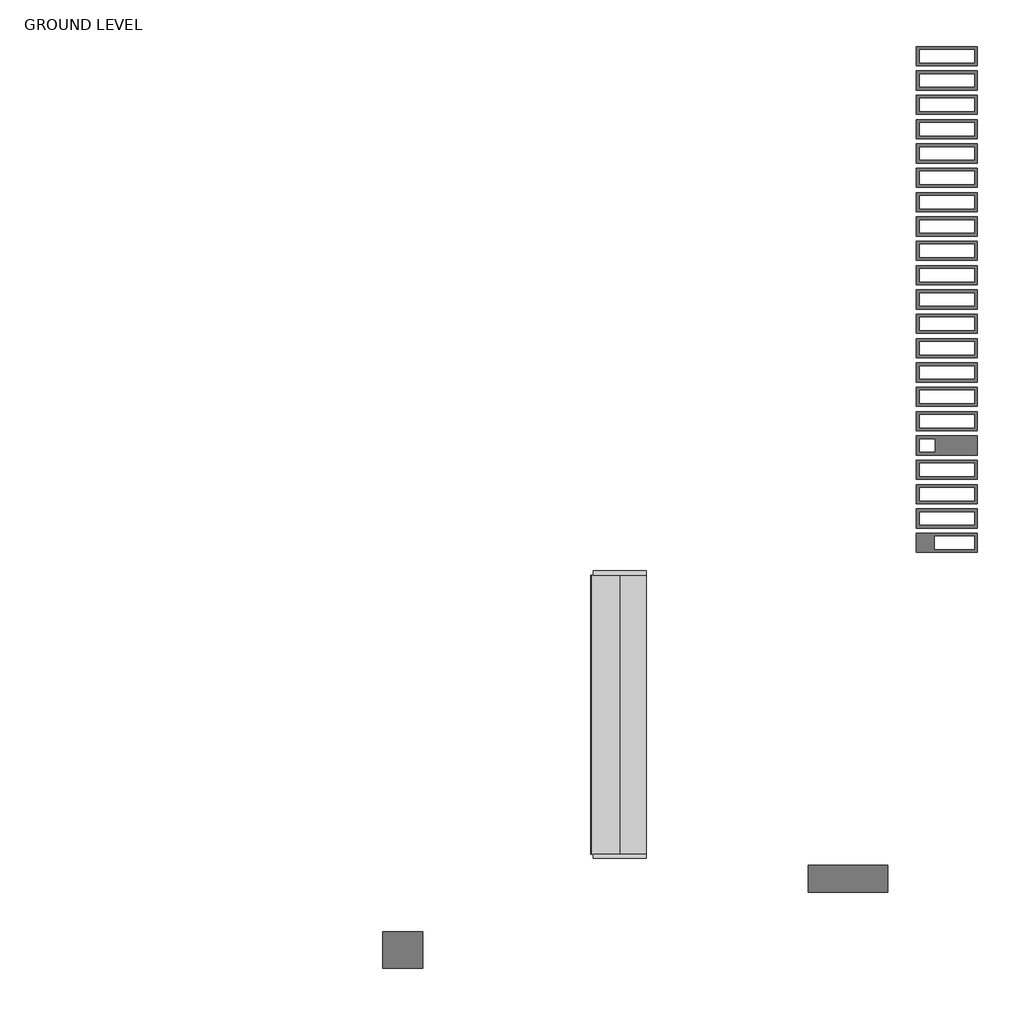
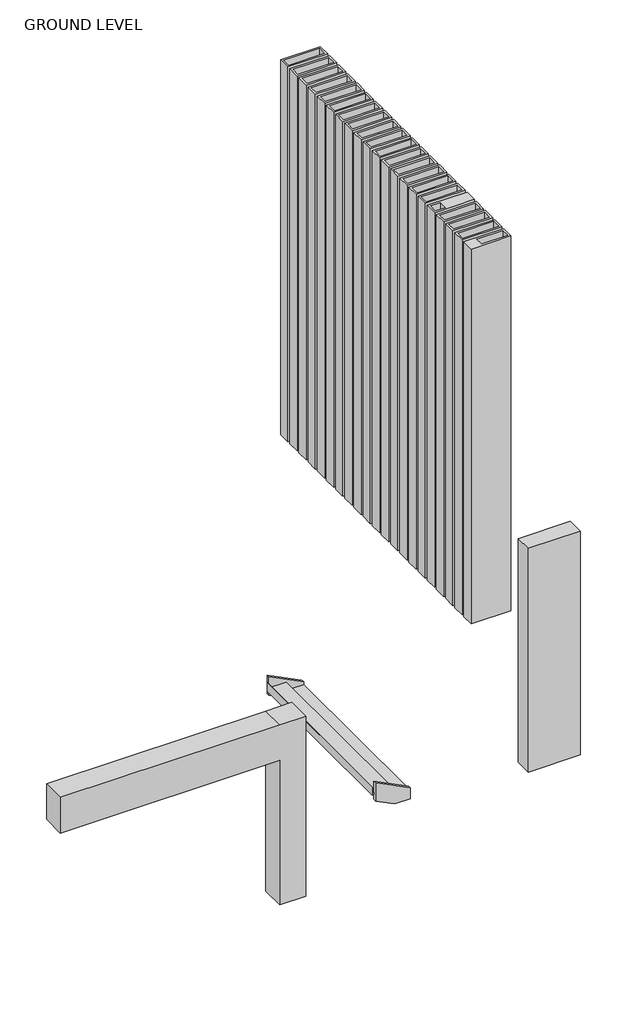
# One storey: 3 proxies, 2 members, 1 stair flight.
"""IFC4 building model written with IfcOpenShell, lengths in millimetres."""

from ifc_helpers import new_model, si_unit, frame, origin, place, context, project, spatial, polyline, outline, extrude, transform, mapped, element, save
from components import generic_models_1_generic_models_1_e82ef2ba, generic_models_6_generic_models_6_c23547c4, model_in_place_1_model_in_place_1_9ea038c9, stair_flight_52a2f54b

model = new_model("IFC4")

# Units and contexts
model_context = context("Model", 3, world=origin())
ifc_project = project(units=[si_unit("LENGTHUNIT", "METRE", prefix="MILLI")], contexts=[model_context])

# Site, building, storey
site = spatial("IfcSite", under=ifc_project)
building = spatial("IfcBuilding", under=site)
storey = spatial("IfcBuildingStorey", under=building, Name="GROUND LEVEL", Elevation=0.0)

# Proxies
placement = place(None, origin())
generic_models_1_generic_models_1_shape = generic_models_1_generic_models_1_e82ef2ba(model_context)
element("IfcBuildingElementProxy", 1, Name="Generic Models 1 : Generic Models 1", ObjectType="Generic Models 1 : Generic Models 1", at=placement, inside=storey, context=model_context, shape_type="MappedRepresentation", body=[
    mapped(generic_models_1_generic_models_1_shape, transform((0.0, 0.0, 0.0), x_axis=(1.0, 0.0, 0.0), y_axis=(0.0, 1.0, 0.0), z_axis=(0.0, 0.0, 1.0))),
])
generic_models_6_generic_models_6_shape = generic_models_6_generic_models_6_c23547c4(model_context)
element("IfcBuildingElementProxy", 2, Name="Generic Models 6 : Generic Models 6", ObjectType="Generic Models 6 : Generic Models 6", at=placement, inside=storey, context=model_context, shape_type="MappedRepresentation", body=[
    mapped(generic_models_6_generic_models_6_shape, transform((0.0, 0.0, 0.0), x_axis=(1.0, 0.0, 0.0), y_axis=(0.0, 1.0, 0.0), z_axis=(0.0, 0.0, 1.0))),
])
model_in_place_1_model_in_place_1_shape = model_in_place_1_model_in_place_1_9ea038c9(model_context)
element("IfcBuildingElementProxy", 3, Name="MODEL IN PLACE 1 : MODEL IN PLACE 1", ObjectType="MODEL IN PLACE 1 : MODEL IN PLACE 1", at=placement, inside=storey, context=model_context, shape_type="MappedRepresentation", body=[
    mapped(model_in_place_1_model_in_place_1_shape, transform((0.0, 0.0, 0.0), x_axis=(1.0, 0.0, 0.0), y_axis=(0.0, 1.0, 0.0), z_axis=(0.0, 0.0, 1.0))),
])

# Members
element("IfcMember", 4, ObjectType="Stringer - 2\" Width", at=placement, inside=storey, context=model_context, shape_type="SweptSolid", body=[
    extrude(outline(polyline([(0.0, -7537.7960918), (203.1066015, -7537.7960918), (507.9066015, -8147.3960918), (167.1298417, -8147.3960918), (0.0, -7813.1364083), (0.0, -7537.7960918)])), frame((0.0, -11453.9453012, 0.0), z_axis=(0.0, 1.0, 0.0), x_axis=(0.0, 0.0, 1.0)), (0.0, 0.0, 1.0), 50.8),
])
element("IfcMember", 5, ObjectType="Stringer - 2\" Width", at=placement, inside=storey, context=model_context, shape_type="SweptSolid", body=[
    extrude(outline(polyline([(0.0, -7537.7960918), (203.1066015, -7537.7960918), (507.9066015, -8147.3960918), (167.1298417, -8147.3960918), (0.0, -7813.1364083), (0.0, -7537.7960918)])), frame((0.0, -8203.7830995, 0.0), z_axis=(0.0, 1.0, 0.0), x_axis=(0.0, 0.0, 1.0)), (0.0, 0.0, 1.0), 50.8),
])

# Stair flight
stair_flight_shape = stair_flight_52a2f54b(model_context)
element("IfcStairFlight", 6, ObjectType="2\" Tread 1\" Nosing 1/4\" Riser", at=placement, inside=storey, context=model_context, shape_type="MappedRepresentation", body=[
    mapped(stair_flight_shape, transform((0.0, 0.0, 0.0), x_axis=(1.0, 0.0, 0.0), y_axis=(0.0, 1.0, 0.0), z_axis=(0.0, 0.0, 1.0))),
])

save(model, "model.ifc")

# Revit data of these elements
# Element 1 (IfcBuildingElementProxy, "Generic Models 1 : Generic Models 1")
#   Phase Created = New Construction
#   Materials on its faces: "GREY COLOUR FRAME"
# Element 2 (IfcBuildingElementProxy, "Generic Models 6 : Generic Models 6")
#   Phase Created = New Construction
#   Materials on its faces: "GREY COLOUR FRAME(2)"
# Element 3 (IfcBuildingElementProxy, "MODEL IN PLACE 1 : MODEL IN PLACE 1")
#   Phase Created = New Construction
# Element 4 (IfcMember, "Stringer - 2\" Width")
#   Phase Created = New Construction
#   Materials on its faces: "MARBLE FLOORING 1'"
# Element 5 (IfcMember, "Stringer - 2\" Width")
#   Phase Created = New Construction
# Element 6 (IfcStairFlight, "2\" Tread 1\" Nosing 1/4\" Riser")
#   Phase Created = New Construction
#   Materials on its faces: "MARBLE FLOORING 1'"
# Materials
#   "GREY COLOUR FRAME": class "Generic", colour RGB 120 120 120, transparency 0, Cost = 0
#   "GREY COLOUR FRAME(2)": class "Generic", colour RGB 120 120 120, transparency 0, Cost = 0
#   "MARBLE FLOORING 1'": class "Generic", colour RGB 120 120 120, transparency 0, Cost = 0
